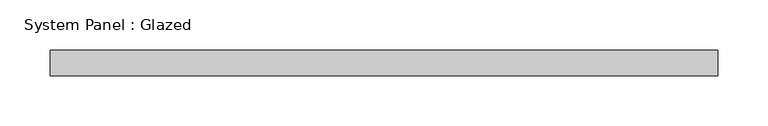
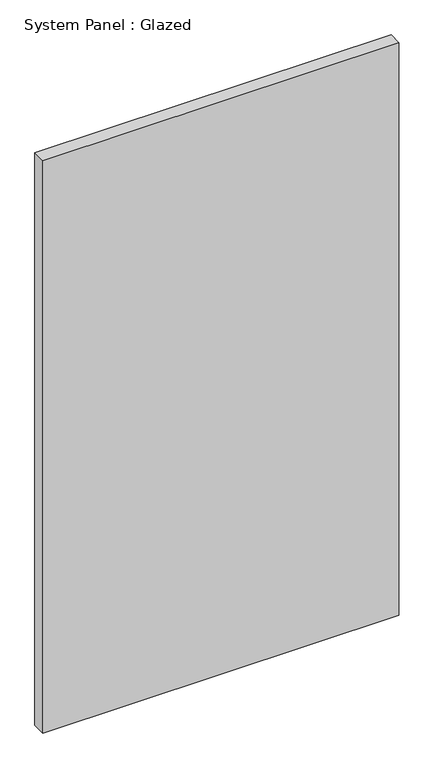
"""IFC4 building model written with IfcOpenShell, lengths in millimetres: plate geometry, System Panel : Glazed."""

from ifc_helpers import new_model, si_unit, origin, origin_with_axes, place, context, project, spatial, polyline, outline, extrude, source, transform, mapped, element, save


def system_panel_glazed_960ffd39(model_context):
    return source(origin(), model_context, "Body", "SweptSolid", [
        extrude(outline(polyline([(333.375, 19.05), (-333.375, 19.05), (-333.375, 44.45), (333.375, 44.45), (333.375, 19.05)])), origin_with_axes(), (0.0, 0.0, 1.0), 1133.0620128),
    ])


if __name__ == "__main__":
    model = new_model("IFC4")
    model_context = context("Model", 3, world=origin())
    ifc_project = project(units=[si_unit("LENGTHUNIT", "METRE", prefix="MILLI")], contexts=[model_context])
    site = spatial("IfcSite", under=ifc_project)
    building = spatial("IfcBuilding", under=site)
    placement = place(None, origin())
    system_panel_glazed_shape = system_panel_glazed_960ffd39(model_context)
    element("IfcPlate", 1, ObjectType="System Panel : Glazed", at=placement, inside=building, context=model_context, shape_type="MappedRepresentation", body=[
        mapped(system_panel_glazed_shape, transform((0.0, 0.0, 0.0), x_axis=(1.0, 0.0, 0.0), y_axis=(0.0, 1.0, 0.0), z_axis=(0.0, 0.0, 1.0))),
    ])
    save(model, "model.ifc")

# Revit data of these elements
# Type "System Panel : Glazed"
#   Construction Type Id = "GSP4R"
#   Analytic Construction = "1/8 in Pilkington single glazing"
#   Visual Light Transmittance = 0.9
#   Solar Heat Gain Coefficient = 0.86
#   Heat Transfer Coefficient (U) = 1.18115 BTU/(h·ft²·°F)
#   Define Thermal Properties by = 1
# Element 1 (IfcPlate, "System Panel : Glazed")
#   Materials on its faces: "Glass"
# Materials
#   "Glass": class "Glass", colour RGB 0 128 192, transparency 0.75, Description = "Soda Lime Glass", Cost = 0
